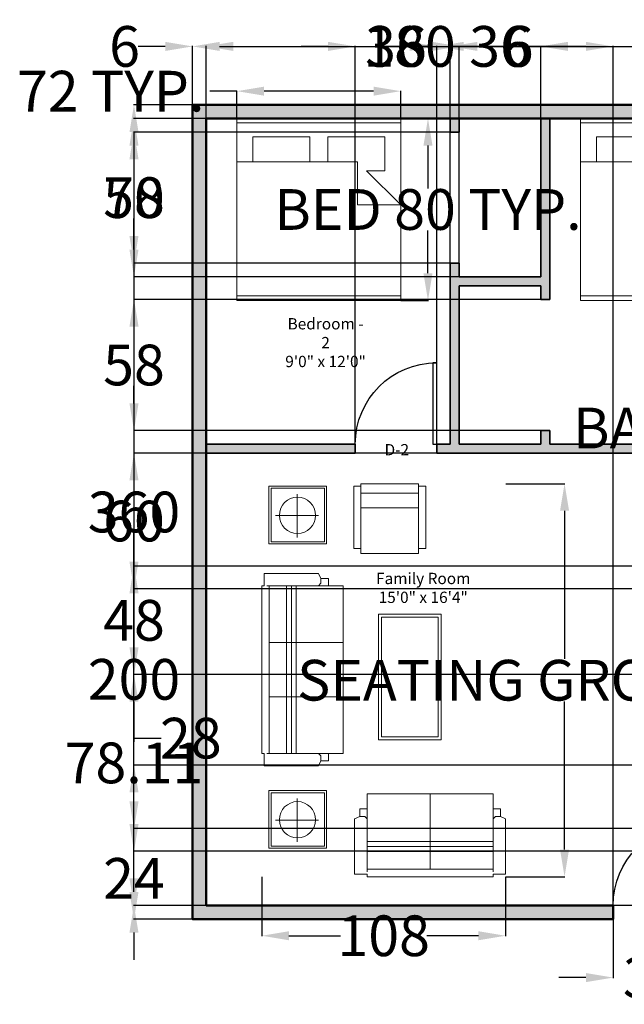
# Model space of a CAD drawing. Units: inches. Extents: x -478 to 256, y -93 to 343.
# Tile 1 of 5: x -478 to -211, y -93 to 343. Entities that reach past the tile are written whole.
import ezdxf

# ---------------------------------------------------------------- set-up
doc = ezdxf.new("R2010")
doc.units = ezdxf.units.IN
for name, color, linetype, lineweight in [('A-ANNO-DIMS', 2, 'Continuous', 18), ('A-ANNO-TEXT', 7, 'Continuous', 18), ('A-AREA-IDEN', 7, 'Continuous', 18), ('A-DOOR', 3, 'Continuous', 25), ('A-WALL-PATT', 8, 'Continuous', 13), ('Furniture', 2, 'Continuous', 18), ('Inner Wall', 5, 'Continuous', 35), ('Outer Wall', 1, 'Continuous', 50)]:
    doc.layers.add(name, color=color, linetype=linetype, lineweight=lineweight)
doc.styles.get("Standard").update_dxf_attribs({"font": 'arial.ttf'})
doc.dimstyles.get("Standard").update_dxf_attribs({"dimtxt": 18, "dimasz": 12, "dimexe": 0.18, "dimexo": 0.0625, "dimgap": 0.09, "dimtad": 0, "dimtih": 1, "dimtoh": 1, "dimdec": 0, "dimzin": 0, "dimdsep": 46, "dimlunit": 3, "dimtxsty": 'Standard', "dimcen": 0.09, "dimadec": 0, "dimazin": 0, "dimtfac": 1, "dimtdec": 0, "dimtofl": 0, "dimtmove": 0, "dimatfit": 3, "dimfxl": 1, "dimtolj": 1, "dimtzin": 0, "dimarcsym": 0})

# ---------------------------------------------------------------- blocks, each defined once
blk = doc.blocks.new('*U2')
for p, q in [((0, 0), (0, -4)), ((36, 0), (36, -4))]:
    blk.add_line(p, q)
blk.add_lwpolyline([(0, 0), (0, 36), (1.75, 36), (1.75, 0)], close=True)
blk.add_arc((0, 0), 36, 0, 90)
blk = doc.blocks.new('KING-00')
for p, q in [((-0.897, -0.947), (-0.897, 0.882)), ((0.602, 0.882), (0.602, -0.464)), ((1.034, -0.947), (1.034, 0.882)), ((0.602, 0.704), (0.881, 0.704)), ((0.881, 0.069), (0.881, 0.704)), ((0.602, 0.069), (0.881, 0.069)), ((0.881, -0.134), (0.602, -0.134)), ((0.881, -0.769), (0.881, -0.134)), ((0.119, -0.464), (0.119, -0.947)), ((0.602, -0.464), (0.119, -0.464)), ((0.119, -0.947), (0.5, -0.566)), ((0.5, -0.769), (0.5, -0.566)), ((0.5, -0.769), (0.881, -0.769))]:
    blk.add_line(p, q)
blk.add_lwpolyline([(-0.948, -0.947), (-0.948, 0.882), (1.084, 0.882), (1.084, -0.947)], close=True)
blk = doc.blocks.new('A$C518662A7')
for p, q in [((24.2, 2257.5), (574.2, 2257.5)), ((24.2, 1707.5), (24.2, 2257.5)), ((574.2, 2257.5), (574.2, 1707.5)), ((2927.5, 2257.5), (3477.5, 2257.5)), ((2927.5, 1707.5), (2927.5, 2257.5)), ((3477.5, 2257.5), (3477.5, 1707.5)), ((44.2, 2237.5), (554.2, 2237.5)), ((44.2, 1727.5), (44.2, 2237.5)), ((304.4, 2193.4), (304.4, 1783.3)), ((554.2, 2237.5), (554.2, 1727.5)), ((2947.5, 2237.5), (3457.5, 2237.5)), ((2947.5, 1727.5), (2947.5, 2237.5)), ((3207.6, 2193.4), (3207.6, 1783.3)), ((3457.5, 2237.5), (3457.5, 1727.5)), ((100.6, 1987.3), (512.6, 1987.3)), ((3003.8, 1987.3), (3415.8, 1987.3)), ((574.2, 1707.5), (24.2, 1707.5)), ((554.2, 1727.5), (44.2, 1727.5)), ((3477.5, 1707.5), (2927.5, 1707.5)), ((3457.5, 1727.5), (2947.5, 1727.5)), ((1243.6, 1213.6), (2443.6, 1213.6)), ((1243.6, 613.6), (1243.6, 1213.6)), ((1273.6, 1183.6), (2413.6, 1183.6)), ((1273.6, 643.6), (1273.6, 1183.6)), ((2413.6, 1183.6), (2413.6, 643.6)), ((2443.6, 1213.6), (2443.6, 613.6)), ((2443.6, 613.6), (1243.6, 613.6)), ((2413.6, 643.6), (1273.6, 643.6))]:
    blk.add_line(p, q)
at = {"linetype": 'ByBlock'}
for p, q in [((855.8, 2302.4), (973.4, 2302.4)), ((855.8, 1784.8), (855.8, 2302.4)), ((973.4, 2326), (2573.4, 2326)), ((973.4, 2302.4), (973.4, 2326)), ((973.4, 1784.8), (973.4, 2278.9)), ((973.4, 2255.4), (2573.4, 2255.4)), ((1514.6, 1549.5), (1514.6, 2255.4)), ((2032.3, 1549.5), (2032.3, 2255.4)), ((2573.4, 2326), (2573.4, 2302.4)), ((2573.4, 2302.4), (2691.1, 2302.4)), ((2573.4, 1784.8), (2573.4, 2278.9)), ((2691.1, 2302.4), (2691.1, 1784.8)), ((2573.4, 2090.7), (973.4, 2090.7)), ((2573.4, 2043.6), (973.4, 2043.6)), ((2573.4, 1996.5), (973.4, 1996.5)), ((902.9, 1761.3), (855.8, 1784.8)), ((949.9, 1761.3), (973.4, 1784.8)), ((973.4, 1690.7), (973.4, 1784.8)), ((2573.4, 1690.7), (2573.4, 1784.8)), ((2597, 1761.3), (2573.4, 1784.8)), ((2691.1, 1784.8), (2644, 1761.3)), ((902.9, 1761.3), (949.9, 1761.3)), ((902.9, 1690.7), (902.9, 1761.3)), ((973.4, 1690.7), (902.9, 1690.7)), ((973.4, 1549.5), (973.4, 1690.7)), ((2644, 1690.7), (2573.4, 1690.7)), ((2573.4, 1690.7), (2573.4, 1549.5)), ((2644, 1761.3), (2597, 1761.3)), ((2644, 1761.3), (2644, 1690.7)), ((2573.4, 1549.5), (973.4, 1549.5)), ((22.9, 1448.9), (22.9, 1380.2)), ((618.7, 1448.9), (22.9, 1448.9)), ((618.7, 1380.2), (618.7, 1448.9)), ((3173, 1392), (3197, 1440)), ((3197, 1440), (3725, 1440)), ((3725, 1440), (3725, 1320)), ((0, 1380.2), (0, 830.2)), ((664.6, 1380.2), (0, 1380.2)), ((91.7, 1380.2), (91.7, 830.2)), ((229.2, 830.2), (229.2, 1380.2)), ((664.6, 830.2), (664.6, 1380.2)), ((2957, 1320), (3101, 1320)), ((2957, 120), (2957, 1320)), ((3101, 1320), (3101, 1392)), ((3101, 1392), (3173, 1392)), ((3101, 1320), (3197, 1320)), ((3173, 1392), (3173, 1344)), ((3173, 1344), (3197, 1320)), ((3197, 1320), (3701, 1320)), ((3413, 120), (3413, 1320)), ((3461, 120), (3461, 1320)), ((3509, 120), (3509, 1320)), ((3677, 1320), (3677, 120)), ((3725, 1320), (3749, 1320)), ((3749, 1320), (3749, 120)), ((0, 830.2), (664.6, 830.2)), ((22.9, 830.2), (22.9, 761.4)), ((22.9, 761.4), (618.7, 761.4)), ((618.7, 761.4), (618.7, 830.2)), ((2957, 720), (3677, 720)), ((3101, 120), (2957, 120)), ((3101, 120), (3197, 120)), ((3101, 48), (3101, 120)), ((3173, 96), (3197, 120)), ((3173, 48), (3173, 96)), ((3197, 120), (3701, 120)), ((3749, 120), (3725, 120)), ((3725, 120), (3725, 0)), ((3173, 48), (3101, 48)), ((3197, 0), (3173, 48)), ((3725, 0), (3197, 0))]:
    blk.add_line(p, q, dxfattribs=at)
for centre in [(302.2, 1985.1), (3205.4, 1985.1)]:
    blk.add_circle(centre, 173.1)
blk = doc.blocks.new('*U14')
for p, q in [((0, 0), (0, -6)), ((36, 0), (36, -6))]:
    blk.add_line(p, q)
blk.add_lwpolyline([(0, 0), (0, 36), (1.75, 36), (1.75, 0)], close=True)
blk.add_arc((0, 0), 36, 0, 90)
blk = doc.blocks.new('*D15')
at = {"layer": 'A-ANNO-DIMS', "color": 0, "lineweight": -2, "transparency": 16777216}
for p, q in [((-309.72, 298.84), (-297.53, 298.84)), ((-297.71, 286.84), (-297.71, 267.89)), ((-297.71, 230.37), (-297.71, 249.32)), ((-309.72, 218.37), (-297.53, 218.37))]:
    blk.add_line(p, q, dxfattribs=at)
at = {"layer": 'A-ANNO-DIMS', "color": 0, "transparency": 16777216}
for points in [[(-299.71, 286.84), (-295.71, 286.84), (-297.71, 298.84)], [(-299.71, 230.37), (-295.71, 230.37), (-297.71, 218.37)]]:
    blk.add_solid(points, dxfattribs=at)
at = {"layer": 'Defpoints', "color": 0, "transparency": 16777216}
for p in [(-309.78, 298.84), (-297.71, 298.84), (-309.78, 218.37)]:
    blk.add_point(p, dxfattribs=at)
at = {"layer": 'A-ANNO-DIMS', "color": 0, "transparency": 16777216, "insert": (-297.71, 258.6), "char_height": 18, "attachment_point": 5}
blk.add_mtext('\\A1;BED 80 TYP.', dxfattribs=at)
blk = doc.blocks.new('*D16')
at = {"layer": 'A-ANNO-DIMS', "color": 0, "lineweight": -2, "transparency": 16777216}
for p, q in [((-382.2, 310.91), (-394.2, 310.91)), ((-382.2, 298.9), (-382.2, 311.09)), ((-321.78, 310.91), (-370.2, 310.91)), ((-309.78, 298.9), (-309.78, 311.09))]:
    blk.add_line(p, q, dxfattribs=at)
at = {"layer": 'A-ANNO-DIMS', "color": 0, "transparency": 16777216}
for points in [[(-370.2, 312.91), (-370.2, 308.91), (-382.2, 310.91)], [(-321.78, 312.91), (-321.78, 308.91), (-309.78, 310.91)]]:
    blk.add_solid(points, dxfattribs=at)
at = {"layer": 'Defpoints', "color": 0, "transparency": 16777216}
for p in [(-382.2, 310.91), (-382.2, 298.84), (-309.78, 298.84)]:
    blk.add_point(p, dxfattribs=at)
at = {"layer": 'A-ANNO-DIMS', "color": 0, "transparency": 16777216, "insert": (-438.03, 310.91), "char_height": 18, "attachment_point": 5}
blk.add_mtext('\\A1;72 TYP.', dxfattribs=at)
blk = doc.blocks.new('*D25')
at = {"layer": 'A-ANNO-DIMS', "color": 0, "lineweight": -2, "transparency": 16777216}
for p, q in [((-116.04, 214.73), (-116.04, 226.73)), ((-118.49, 202.73), (-115.86, 202.73)), ((-118.49, 185.95), (-115.86, 185.95)), ((-116.04, 173.95), (-116.04, 161.95)), ((-116.04, 161.95), (-128.04, 161.95))]:
    blk.add_line(p, q, dxfattribs=at)
at = {"layer": 'A-ANNO-DIMS', "color": 0, "transparency": 16777216}
for points in [[(-118.04, 214.73), (-114.04, 214.73), (-116.04, 202.73)], [(-118.04, 173.95), (-114.04, 173.95), (-116.04, 185.95)]]:
    blk.add_solid(points, dxfattribs=at)
at = {"layer": 'Defpoints', "color": 0, "transparency": 16777216}
for p in [(-118.56, 202.73), (-118.56, 185.95), (-116.04, 185.95)]:
    blk.add_point(p, dxfattribs=at)
at = {"layer": 'A-ANNO-DIMS', "color": 0, "transparency": 16777216, "insert": (-181.85, 161.95), "char_height": 18, "attachment_point": 5}
blk.add_mtext('\\A1;BASIN 17', dxfattribs=at)
blk = doc.blocks.new('*D29')
at = {"layer": 'A-ANNO-DIMS', "color": 0, "lineweight": -2, "transparency": 16777216}
for p, q in [((-263.32, 137.36), (-237.13, 137.36)), ((-237.31, 125.36), (-237.31, 59.86)), ((-237.31, -24.45), (-237.31, 41.05)), ((-263.32, -36.45), (-237.13, -36.45))]:
    blk.add_line(p, q, dxfattribs=at)
at = {"layer": 'A-ANNO-DIMS', "color": 0, "transparency": 16777216}
for points in [[(-239.31, 125.36), (-235.31, 125.36), (-237.31, 137.36)], [(-239.31, -24.45), (-235.31, -24.45), (-237.31, -36.45)]]:
    blk.add_solid(points, dxfattribs=at)
at = {"layer": 'Defpoints', "color": 0, "transparency": 16777216}
for p in [(-263.38, 137.36), (-263.38, -36.45), (-237.31, -36.45)]:
    blk.add_point(p, dxfattribs=at)
at = {"layer": 'A-ANNO-DIMS', "color": 0, "transparency": 16777216, "insert": (-237.31, 50.46), "char_height": 18, "attachment_point": 5}
blk.add_mtext('\\A1;SEATING GROUP 174', dxfattribs=at)
blk = doc.blocks.new('*D30')
at = {"layer": 'A-ANNO-DIMS', "color": 0, "lineweight": -2, "transparency": 16777216}
for p, q in [((-371.22, -36.51), (-371.22, -62.7)), ((-263.38, -36.51), (-263.38, -62.7)), ((-359.22, -62.52), (-336.45, -62.52)), ((-275.38, -62.52), (-298.15, -62.52))]:
    blk.add_line(p, q, dxfattribs=at)
at = {"layer": 'A-ANNO-DIMS', "color": 0, "transparency": 16777216}
for points in [[(-359.22, -60.52), (-359.22, -64.52), (-371.22, -62.52)], [(-275.38, -60.52), (-275.38, -64.52), (-263.38, -62.52)]]:
    blk.add_solid(points, dxfattribs=at)
at = {"layer": 'Defpoints', "color": 0, "transparency": 16777216}
for p in [(-371.22, -36.45), (-263.38, -36.45), (-371.22, -62.52)]:
    blk.add_point(p, dxfattribs=at)
at = {"layer": 'A-ANNO-DIMS', "color": 0, "transparency": 16777216, "insert": (-317.3, -62.52), "char_height": 18, "attachment_point": 5}
blk.add_mtext('\\A1;108', dxfattribs=at)
blk = doc.blocks.new('*D31')
at = {"layer": 'A-ANNO-DIMS', "color": 0, "lineweight": -2, "transparency": 16777216}
for p, q in [((-401.86, 304.9), (-401.86, 330.89)), ((78.14, 304.9), (78.14, 330.89)), ((-389.86, 330.71), (-182.16, 330.71)), ((66.14, 330.71), (-141.55, 330.71))]:
    blk.add_line(p, q, dxfattribs=at)
at = {"layer": 'A-ANNO-DIMS', "color": 0, "transparency": 16777216}
for points in [[(-389.86, 332.71), (-389.86, 328.71), (-401.86, 330.71)], [(66.14, 332.71), (66.14, 328.71), (78.14, 330.71)]]:
    blk.add_solid(points, dxfattribs=at)
at = {"layer": 'Defpoints', "color": 0, "transparency": 16777216}
for p in [(78.14, 330.71), (-401.86, 304.84), (78.14, 304.84)]:
    blk.add_point(p, dxfattribs=at)
at = {"layer": 'A-ANNO-DIMS', "color": 0, "transparency": 16777216, "insert": (-161.86, 330.71), "char_height": 18, "attachment_point": 5}
blk.add_mtext('\\A1;480', dxfattribs=at)
blk = doc.blocks.new('*D32')
at = {"layer": 'A-ANNO-DIMS', "color": 0, "lineweight": -2, "transparency": 16777216}
for p, q in [((-401.92, 304.84), (-427.9, 304.84)), ((-427.72, 292.84), (-427.72, 134.13)), ((-427.72, -43.16), (-427.72, 115.55)), ((-401.92, -55.16), (-427.9, -55.16))]:
    blk.add_line(p, q, dxfattribs=at)
at = {"layer": 'A-ANNO-DIMS', "color": 0, "transparency": 16777216}
for points in [[(-429.72, 292.84), (-425.72, 292.84), (-427.72, 304.84)], [(-429.72, -43.16), (-425.72, -43.16), (-427.72, -55.16)]]:
    blk.add_solid(points, dxfattribs=at)
at = {"layer": 'Defpoints', "color": 0, "transparency": 16777216}
for p in [(-427.72, 304.84), (-401.86, 304.84), (-401.86, -55.16)]:
    blk.add_point(p, dxfattribs=at)
at = {"layer": 'A-ANNO-DIMS', "color": 0, "transparency": 16777216, "insert": (-427.72, 124.84), "char_height": 18, "attachment_point": 5}
blk.add_mtext('\\A1;360', dxfattribs=at)
blk = doc.blocks.new('*D33')
at = {"layer": 'A-ANNO-DIMS', "color": 0, "lineweight": -2, "transparency": 16777216}
for p, q in [((-395.86, -49.1), (-395.86, 330.89)), ((-215.86, -49.1), (-215.86, 330.89)), ((-383.86, 330.71), (-324.95, 330.71)), ((-227.86, 330.71), (-286.76, 330.71))]:
    blk.add_line(p, q, dxfattribs=at)
at = {"layer": 'A-ANNO-DIMS', "color": 0, "transparency": 16777216}
for points in [[(-383.86, 332.71), (-383.86, 328.71), (-395.86, 330.71)], [(-227.86, 332.71), (-227.86, 328.71), (-215.86, 330.71)]]:
    blk.add_solid(points, dxfattribs=at)
at = {"layer": 'Defpoints', "color": 0, "transparency": 16777216}
for p in [(-215.86, 330.71), (-395.86, -49.16), (-215.86, -49.16)]:
    blk.add_point(p, dxfattribs=at)
at = {"layer": 'A-ANNO-DIMS', "color": 0, "transparency": 16777216, "insert": (-305.86, 330.71), "char_height": 18, "attachment_point": 5}
blk.add_mtext('\\A1;180', dxfattribs=at)
blk = doc.blocks.new('*D34')
at = {"layer": 'A-ANNO-DIMS', "color": 0, "lineweight": -2, "transparency": 16777216}
for p, q in [((-215.855811, -55.221403), (-215.855811, -81.203903)), ((-179.855811, -55.221403), (-179.855811, -81.203903)), ((-227.855811, -81.023903), (-239.855811, -81.023903)), ((-167.855811, -81.023903), (-155.855811, -81.023903))]:
    blk.add_line(p, q, dxfattribs=at)
at = {"layer": 'A-ANNO-DIMS', "color": 0, "transparency": 16777216}
for points in [[(-227.855811, -79.023903), (-227.855811, -83.023903), (-215.855811, -81.023903)], [(-167.855811, -79.023903), (-167.855811, -83.023903), (-179.855811, -81.023903)]]:
    blk.add_solid(points, dxfattribs=at)
at = {"layer": 'Defpoints', "color": 0, "transparency": 16777216}
for p in [(-215.855811, -55.158903), (-179.855811, -55.158903), (-179.855811, -81.023903)]:
    blk.add_point(p, dxfattribs=at)
at = {"layer": 'A-ANNO-DIMS', "color": 0, "transparency": 16777216, "insert": (-197.855811, -81.023903), "char_height": 18, "attachment_point": 5}
blk.add_mtext('\\A1;36', dxfattribs=at)
blk = doc.blocks.new('*D36')
at = {"layer": 'A-ANNO-DIMS', "color": 0, "lineweight": -2, "transparency": 16777216}
for p, q in [((-395.92, 150.84), (-427.9, 150.84)), ((-427.72, 138.84), (-427.72, 60.12)), ((-427.72, -37.16), (-427.72, 41.56)), ((-395.92, -49.16), (-427.9, -49.16))]:
    blk.add_line(p, q, dxfattribs=at)
at = {"layer": 'A-ANNO-DIMS', "color": 0, "transparency": 16777216}
for points in [[(-429.72, 138.84), (-425.72, 138.84), (-427.72, 150.84)], [(-429.72, -37.16), (-425.72, -37.16), (-427.72, -49.16)]]:
    blk.add_solid(points, dxfattribs=at)
at = {"layer": 'Defpoints', "color": 0, "transparency": 16777216}
for p in [(-427.72, 150.84), (-395.86, 150.84), (-395.86, -49.16)]:
    blk.add_point(p, dxfattribs=at)
at = {"layer": 'A-ANNO-DIMS', "color": 0, "transparency": 16777216, "insert": (-427.72, 50.84), "char_height": 18, "attachment_point": 5}
blk.add_mtext('\\A1;200', dxfattribs=at)
blk = doc.blocks.new('*D37')
at = {"layer": 'A-ANNO-DIMS', "color": 0, "lineweight": -2, "transparency": 16777216}
for p, q in [((-283.855811, 228.903597), (-283.855811, 330.886097)), ((-247.855811, 228.903597), (-247.855811, 330.886097)), ((-295.855811, 330.706097), (-307.855811, 330.706097)), ((-235.855811, 330.706097), (-223.855811, 330.706097))]:
    blk.add_line(p, q, dxfattribs=at)
at = {"layer": 'A-ANNO-DIMS', "color": 0, "transparency": 16777216}
for points in [[(-295.855811, 332.706097), (-295.855811, 328.706097), (-283.855811, 330.706097)], [(-235.855811, 332.706097), (-235.855811, 328.706097), (-247.855811, 330.706097)]]:
    blk.add_solid(points, dxfattribs=at)
at = {"layer": 'Defpoints', "color": 0, "transparency": 16777216}
for p in [(-247.855811, 330.706097), (-283.855811, 228.841097), (-247.855811, 228.841097)]:
    blk.add_point(p, dxfattribs=at)
at = {"layer": 'A-ANNO-DIMS', "color": 0, "transparency": 16777216, "insert": (-265.855811, 330.706097), "char_height": 18, "attachment_point": 5}
blk.add_mtext('\\A1;36', dxfattribs=at)
blk = doc.blocks.new('*D38')
at = {"layer": 'A-ANNO-DIMS', "color": 0, "lineweight": -2, "transparency": 16777216}
for p, q in [((-247.92, 298.84), (-427.9, 298.84)), ((-427.72, 286.84), (-427.72, 273.12)), ((-427.72, 240.84), (-427.72, 254.56)), ((-247.92, 228.84), (-427.9, 228.84))]:
    blk.add_line(p, q, dxfattribs=at)
at = {"layer": 'A-ANNO-DIMS', "color": 0, "transparency": 16777216}
for points in [[(-429.72, 286.84), (-425.72, 286.84), (-427.72, 298.84)], [(-429.72, 240.84), (-425.72, 240.84), (-427.72, 228.84)]]:
    blk.add_solid(points, dxfattribs=at)
at = {"layer": 'Defpoints', "color": 0, "transparency": 16777216}
for p in [(-427.72, 298.84), (-247.86, 298.84), (-247.86, 228.84)]:
    blk.add_point(p, dxfattribs=at)
at = {"layer": 'A-ANNO-DIMS', "color": 0, "transparency": 16777216, "insert": (-427.72, 263.84), "char_height": 18, "attachment_point": 5}
blk.add_mtext('\\A1;70', dxfattribs=at)
blk = doc.blocks.new('*D42')
at = {"layer": 'A-ANNO-DIMS', "color": 0, "lineweight": -2, "transparency": 16777216}
for p, q in [((-329.855811, 154.903597), (-329.855811, 330.886097)), ((-293.855811, 154.903597), (-293.855811, 330.886097)), ((-341.855811, 330.706097), (-353.855811, 330.706097)), ((-281.855811, 330.706097), (-269.855811, 330.706097))]:
    blk.add_line(p, q, dxfattribs=at)
at = {"layer": 'A-ANNO-DIMS', "color": 0, "transparency": 16777216}
for points in [[(-341.855811, 332.706097), (-341.855811, 328.706097), (-329.855811, 330.706097)], [(-281.855811, 332.706097), (-281.855811, 328.706097), (-293.855811, 330.706097)]]:
    blk.add_solid(points, dxfattribs=at)
at = {"layer": 'Defpoints', "color": 0, "transparency": 16777216}
for p in [(-293.855811, 330.706097), (-329.855811, 154.841097), (-293.855811, 154.841097)]:
    blk.add_point(p, dxfattribs=at)
at = {"layer": 'A-ANNO-DIMS', "color": 0, "transparency": 16777216, "insert": (-311.855811, 330.706097), "char_height": 18, "attachment_point": 5}
blk.add_mtext('\\A1;36', dxfattribs=at)
blk = doc.blocks.new('*D43')
at = {"layer": 'A-ANNO-DIMS', "color": 0, "lineweight": -2, "transparency": 16777216}
for p, q in [((-293.86, 154.9), (-293.86, 330.89)), ((-287.86, 154.9), (-287.86, 330.89)), ((-305.86, 330.71), (-317.86, 330.71)), ((-275.86, 330.71), (-263.86, 330.71))]:
    blk.add_line(p, q, dxfattribs=at)
at = {"layer": 'A-ANNO-DIMS', "color": 0, "transparency": 16777216}
for points in [[(-305.86, 332.71), (-305.86, 328.71), (-293.86, 330.71)], [(-275.86, 332.71), (-275.86, 328.71), (-287.86, 330.71)]]:
    blk.add_solid(points, dxfattribs=at)
at = {"layer": 'Defpoints', "color": 0, "transparency": 16777216}
for p in [(-287.86, 330.71), (-293.86, 154.84), (-287.86, 154.84)]:
    blk.add_point(p, dxfattribs=at)
at = {"layer": 'A-ANNO-DIMS', "color": 0, "transparency": 16777216, "insert": (-257.82, 330.71), "char_height": 18, "attachment_point": 5}
blk.add_mtext('\\A1;6', dxfattribs=at)
blk = doc.blocks.new('*D52')
at = {"layer": 'A-ANNO-DIMS', "color": 0, "lineweight": -2, "transparency": 16777216}
for p, q in [((-427.72, 12.84), (-427.72, 24.84)), ((-427.72, 24.84), (-415.72, 24.84)), ((0.08, 12.84), (-427.9, 12.84)), ((-427.72, -3.16), (-427.72, 0.84)), ((0.08, -15.16), (-427.9, -15.16))]:
    blk.add_line(p, q, dxfattribs=at)
at = {"layer": 'A-ANNO-DIMS', "color": 0, "transparency": 16777216}
for points in [[(-429.72, 0.84), (-425.72, 0.84), (-427.72, 12.84)], [(-429.72, -3.16), (-425.72, -3.16), (-427.72, -15.16)]]:
    blk.add_solid(points, dxfattribs=at)
at = {"layer": 'Defpoints', "color": 0, "transparency": 16777216}
for p in [(-427.72, 12.84), (0.14, 12.84), (0.14, -15.16)]:
    blk.add_point(p, dxfattribs=at)
at = {"layer": 'A-ANNO-DIMS', "color": 0, "transparency": 16777216, "insert": (-402.57, 24.84), "char_height": 18, "attachment_point": 5}
blk.add_mtext('\\A1;28', dxfattribs=at)
blk = doc.blocks.new('*D54')
at = {"layer": 'A-ANNO-DIMS', "color": 0, "lineweight": -2, "transparency": 16777216}
for p, q in [((-106.35, 100.95), (-427.9, 100.95)), ((-427.72, 88.95), (-427.72, 86.23)), ((-427.72, 64.95), (-427.72, 67.67)), ((-106.35, 52.95), (-427.9, 52.95))]:
    blk.add_line(p, q, dxfattribs=at)
at = {"layer": 'A-ANNO-DIMS', "color": 0, "transparency": 16777216}
for points in [[(-429.72, 88.95), (-425.72, 88.95), (-427.72, 100.95)], [(-429.72, 64.95), (-425.72, 64.95), (-427.72, 52.95)]]:
    blk.add_solid(points, dxfattribs=at)
at = {"layer": 'Defpoints', "color": 0, "transparency": 16777216}
for p in [(-427.72, 100.95), (-106.28, 100.95), (-106.28, 52.95)]:
    blk.add_point(p, dxfattribs=at)
at = {"layer": 'A-ANNO-DIMS', "color": 0, "transparency": 16777216, "insert": (-427.72, 76.95), "char_height": 18, "attachment_point": 5}
blk.add_mtext('\\A1;48', dxfattribs=at)
blk = doc.blocks.new('*D55')
at = {"layer": 'A-ANNO-DIMS', "color": 0, "lineweight": -2, "transparency": 16777216}
for p, q in [((-401.86, 304.9), (-401.86, 330.89)), ((-395.86, 298.9), (-395.86, 330.89)), ((-413.86, 330.71), (-425.86, 330.71)), ((-383.86, 330.71), (-371.86, 330.71))]:
    blk.add_line(p, q, dxfattribs=at)
at = {"layer": 'A-ANNO-DIMS', "color": 0, "transparency": 16777216}
for points in [[(-413.86, 332.71), (-413.86, 328.71), (-401.86, 330.71)], [(-383.86, 332.71), (-383.86, 328.71), (-395.86, 330.71)]]:
    blk.add_solid(points, dxfattribs=at)
at = {"layer": 'Defpoints', "color": 0, "transparency": 16777216}
for p in [(-401.86, 330.71), (-401.86, 304.84), (-395.86, 298.84)]:
    blk.add_point(p, dxfattribs=at)
at = {"layer": 'A-ANNO-DIMS', "color": 0, "transparency": 16777216, "insert": (-431.89, 330.71), "char_height": 18, "attachment_point": 5}
blk.add_mtext('\\A1;6', dxfattribs=at)
blk = doc.blocks.new('*D58')
at = {"layer": 'A-ANNO-DIMS', "color": 0, "lineweight": -2, "transparency": 16777216}
for p, q in [((-427.720811, -13.158903), (-427.720811, -1.158903)), ((-99.918311, -25.158903), (-427.900811, -25.158903)), ((-99.918311, -49.158903), (-427.900811, -49.158903)), ((-427.720811, -61.158903), (-427.720811, -73.158903))]:
    blk.add_line(p, q, dxfattribs=at)
at = {"layer": 'A-ANNO-DIMS', "color": 0, "transparency": 16777216}
for points in [[(-429.720811, -13.158903), (-425.720811, -13.158903), (-427.720811, -25.158903)], [(-429.720811, -61.158903), (-425.720811, -61.158903), (-427.720811, -49.158903)]]:
    blk.add_solid(points, dxfattribs=at)
at = {"layer": 'Defpoints', "color": 0, "transparency": 16777216}
for p in [(-427.720811, -25.158903), (-99.855811, -25.158903), (-99.855811, -49.158903)]:
    blk.add_point(p, dxfattribs=at)
at = {"layer": 'A-ANNO-DIMS', "color": 0, "transparency": 16777216, "insert": (-427.720811, -37.158903), "char_height": 18, "attachment_point": 5}
blk.add_mtext('\\A1;24', dxfattribs=at)
blk = doc.blocks.new('*D61')
at = {"layer": 'A-ANNO-DIMS', "color": 0, "lineweight": -2, "transparency": 16777216}
for p, q in [((-106.35, 52.95), (-427.9, 52.95)), ((-427.72, 40.95), (-427.72, 23.18)), ((-427.72, -13.16), (-427.72, 4.61)), ((-99.92, -25.16), (-427.9, -25.16))]:
    blk.add_line(p, q, dxfattribs=at)
at = {"layer": 'A-ANNO-DIMS', "color": 0, "transparency": 16777216}
for points in [[(-429.72, 40.95), (-425.72, 40.95), (-427.72, 52.95)], [(-429.72, -13.16), (-425.72, -13.16), (-427.72, -25.16)]]:
    blk.add_solid(points, dxfattribs=at)
at = {"layer": 'Defpoints', "color": 0, "transparency": 16777216}
for p in [(-427.72, 52.95), (-106.28, 52.95), (-99.86, -25.16)]:
    blk.add_point(p, dxfattribs=at)
at = {"layer": 'A-ANNO-DIMS', "color": 0, "transparency": 16777216, "insert": (-427.72, 13.9), "char_height": 18, "attachment_point": 5}
blk.add_mtext('\\A1;78.11', dxfattribs=at)
blk = doc.blocks.new('*D63')
at = {"layer": 'A-ANNO-DIMS', "color": 0, "lineweight": -2, "transparency": 16777216}
for p, q in [((-287.92, 292.84), (-427.9, 292.84)), ((-427.72, 280.84), (-427.72, 273.12)), ((-427.72, 246.84), (-427.72, 254.56)), ((-287.92, 234.84), (-427.9, 234.84))]:
    blk.add_line(p, q, dxfattribs=at)
at = {"layer": 'A-ANNO-DIMS', "color": 0, "transparency": 16777216}
for points in [[(-429.72, 280.84), (-425.72, 280.84), (-427.72, 292.84)], [(-429.72, 246.84), (-425.72, 246.84), (-427.72, 234.84)]]:
    blk.add_solid(points, dxfattribs=at)
at = {"layer": 'Defpoints', "color": 0, "transparency": 16777216}
for p in [(-427.72, 292.84), (-287.86, 292.84), (-287.86, 234.84)]:
    blk.add_point(p, dxfattribs=at)
at = {"layer": 'A-ANNO-DIMS', "color": 0, "transparency": 16777216, "insert": (-427.72, 263.84), "char_height": 18, "attachment_point": 5}
blk.add_mtext('\\A1;58', dxfattribs=at)
blk = doc.blocks.new('*D64')
at = {"layer": 'A-ANNO-DIMS', "color": 0, "lineweight": -2, "transparency": 16777216}
for p, q in [((-247.92, 218.84), (-427.9, 218.84)), ((-427.72, 206.84), (-427.72, 199.12)), ((-427.72, 172.84), (-427.72, 180.56)), ((-247.92, 160.84), (-427.9, 160.84))]:
    blk.add_line(p, q, dxfattribs=at)
at = {"layer": 'A-ANNO-DIMS', "color": 0, "transparency": 16777216}
for points in [[(-429.72, 206.84), (-425.72, 206.84), (-427.72, 218.84)], [(-429.72, 172.84), (-425.72, 172.84), (-427.72, 160.84)]]:
    blk.add_solid(points, dxfattribs=at)
at = {"layer": 'Defpoints', "color": 0, "transparency": 16777216}
for p in [(-427.72, 218.84), (-247.86, 218.84), (-247.86, 160.84)]:
    blk.add_point(p, dxfattribs=at)
at = {"layer": 'A-ANNO-DIMS', "color": 0, "transparency": 16777216, "insert": (-427.72, 189.84), "char_height": 18, "attachment_point": 5}
blk.add_mtext('\\A1;58', dxfattribs=at)
blk = doc.blocks.new('*D66')
at = {"layer": 'A-ANNO-DIMS', "color": 0, "lineweight": -2, "transparency": 16777216}
for p, q in [((24.08, 150.84), (-427.9, 150.84)), ((-427.72, 138.84), (-427.72, 130.12)), ((-427.72, 102.84), (-427.72, 111.56)), ((24.08, 90.84), (-427.9, 90.84))]:
    blk.add_line(p, q, dxfattribs=at)
at = {"layer": 'A-ANNO-DIMS', "color": 0, "transparency": 16777216}
for points in [[(-429.72, 138.84), (-425.72, 138.84), (-427.72, 150.84)], [(-429.72, 102.84), (-425.72, 102.84), (-427.72, 90.84)]]:
    blk.add_solid(points, dxfattribs=at)
at = {"layer": 'Defpoints', "color": 0, "transparency": 16777216}
for p in [(-427.72, 150.84), (24.14, 150.84), (24.14, 90.84)]:
    blk.add_point(p, dxfattribs=at)
at = {"layer": 'A-ANNO-DIMS', "color": 0, "transparency": 16777216, "insert": (-427.72, 120.84), "char_height": 18, "attachment_point": 5}
blk.add_mtext('\\A1;60', dxfattribs=at)
blk = doc.blocks.new('*D68')
at = {"layer": 'A-ANNO-DIMS', "color": 0, "lineweight": -2, "transparency": 16777216}
for p, q in [((-427.720811, -13.158903), (-427.720811, -1.158903)), ((72.081689, -25.158903), (-427.900811, -25.158903)), ((72.081689, -49.158903), (-427.900811, -49.158903)), ((-427.720811, -61.158903), (-427.720811, -73.158903))]:
    blk.add_line(p, q, dxfattribs=at)
at = {"layer": 'A-ANNO-DIMS', "color": 0, "transparency": 16777216}
for points in [[(-429.720811, -13.158903), (-425.720811, -13.158903), (-427.720811, -25.158903)], [(-429.720811, -61.158903), (-425.720811, -61.158903), (-427.720811, -49.158903)]]:
    blk.add_solid(points, dxfattribs=at)
at = {"layer": 'Defpoints', "color": 0, "transparency": 16777216}
for p in [(-427.720811, -25.158903), (72.144189, -25.158903), (72.144189, -49.158903)]:
    blk.add_point(p, dxfattribs=at)
at = {"layer": 'A-ANNO-DIMS', "color": 0, "transparency": 16777216, "insert": (-427.720811, -37.158903), "char_height": 18, "attachment_point": 5}
blk.add_mtext('\\A1;24', dxfattribs=at)

msp = doc.modelspace()

# ---------------------------------------------------------------- hatches: boundary and pattern name
at = {"layer": 'A-WALL-PATT'}
h = msp.add_hatch(color=256, dxfattribs=at)
h.dxf.hatch_style = 1
h.paths.add_polyline_path([(-395.856, 298.841), (72.144, 298.841), (72.144, 20.841), (78.144, 20.841), (78.144, 304.841), (-401.856, 304.841), (-401.856, -55.159), (-215.856, -55.159), (-215.856, -49.159), (-395.856, -49.159)])
h.paths.add_polyline_path([(78.144, -15.159), (72.144, -15.159), (72.144, -49.159), (-179.856, -49.159), (-179.856, -55.159), (78.144, -55.159)], flags=17)
h = msp.add_hatch(color=256, dxfattribs=at)
h.dxf.hatch_style = 1
h.paths.add_polyline_path([(-329.856, 154.841), (-395.856, 154.841), (-395.856, 150.841), (-329.856, 150.841)])
h.paths.add_polyline_path([(-177.856, 154.841), (-243.856, 154.841), (-243.856, 160.841), (-247.856, 160.841), (-247.856, 154.841), (-283.856, 154.841), (-283.856, 224.841), (-247.856, 224.841), (-247.856, 218.841), (-243.856, 218.841), (-243.856, 298.841), (-247.856, 298.841), (-247.856, 228.841), (-283.856, 228.841), (-283.856, 234.841), (-287.856, 234.841), (-287.856, 154.841), (-293.856, 154.841), (-293.856, 150.841), (-177.856, 150.841)])
h.paths.add_polyline_path([(-283.856, 298.841), (-287.856, 298.841), (-287.856, 292.841), (-283.856, 292.841)], flags=17)
h.paths.add_polyline_path([(-131.856, 298.841), (-135.856, 298.841), (-135.856, 154.841), (-141.856, 154.841), (-141.856, 150.841), (-117.856, 150.841), (-117.856, 154.841), (-131.856, 154.841)])
h.paths.add_polyline_path([(-79.856, 298.841), (-83.856, 298.841), (-83.856, 154.841), (-89.856, 154.841), (-89.856, 150.841), (-73.856, 150.841), (-73.856, 154.841), (-79.856, 154.841)])
h.paths.add_polyline_path([(32.144, 154.841), (-33.856, 154.841), (-33.856, 150.841), (-3.856, 150.841), (-3.856, 12.841), (0.144, 12.841), (0.144, 62.841), (72.144, 62.841), (72.144, 66.841), (0.144, 66.841), (0.144, 150.841), (32.144, 150.841)])
h.paths.add_polyline_path([(72.144, 154.841), (60.144, 154.841), (60.144, 150.841), (72.144, 150.841)], flags=17)
h.paths.add_polyline_path([(6.144, -21.159), (0.144, -21.159), (0.144, -15.159), (-3.856, -15.159), (-3.856, -49.159), (0.144, -49.159), (0.144, -25.159), (6.144, -25.159)])
h.paths.add_polyline_path([(72.144, -21.159), (66.144, -21.159), (66.144, -25.159), (72.144, -25.159)])

# ---------------------------------------------------------------- linework, layer by layer
at = {"layer": 'Inner Wall'}
for p, q in [((-287.856, 292.841), (-287.856, 298.841)), ((-283.856, 292.841), (-283.856, 298.841)), ((-247.856, 298.841), (-247.856, 228.841)), ((-243.856, 298.841), (-243.856, 218.841)), ((-287.856, 292.841), (-283.856, 292.841)), ((-287.856, 154.841), (-287.856, 234.841)), ((-287.856, 234.841), (-283.856, 234.841)), ((-283.856, 228.841), (-283.856, 234.841)), ((-283.856, 228.841), (-247.856, 228.841)), ((-283.856, 154.841), (-283.856, 224.841)), ((-283.856, 224.841), (-247.856, 224.841)), ((-247.856, 224.841), (-247.856, 218.841)), ((-247.856, 218.841), (-243.856, 218.841)), ((-247.856, 160.841), (-243.856, 160.841)), ((-247.856, 160.841), (-247.856, 154.841)), ((-243.856, 160.841), (-243.856, 154.841)), ((-395.856, 154.841), (-329.856, 154.841)), ((-329.856, 150.841), (-329.856, 154.841)), ((-293.856, 150.841), (-293.856, 154.841)), ((-293.856, 154.841), (-287.856, 154.841)), ((-283.856, 154.841), (-247.856, 154.841)), ((-243.856, 154.841), (-177.856, 154.841)), ((-395.856, 150.841), (-329.856, 150.841)), ((-293.856, 150.841), (-177.856, 150.841))]:
    msp.add_line(p, q, dxfattribs=at)
at = {"layer": 'Outer Wall'}
for p, q in [((-395.856, 298.841), (72.144, 298.841)), ((-395.856, -49.159), (-395.856, 298.841)), ((-215.856, -49.159), (-395.856, -49.159)), ((-215.856, -55.159), (-215.856, -49.159))]:
    msp.add_line(p, q, dxfattribs=at)
msp.add_lwpolyline([(-215.856, -55.159), (-401.856, -55.159), (-401.856, 304.841), (78.144, 304.841), (78.144, 20.841)], dxfattribs=at)

# ---------------------------------------------------------------- block references
at = {"layer": 'A-DOOR', "xscale": -1}
for name, p in [('*U2', (-293.856, 154.841)), ('*U14', (-179.856, -49.159))]:
    msp.add_blockref(name, p, dxfattribs=at)
at = {"layer": 'Furniture'}
for name, p, xscale, yscale, zscale, rotation in [('KING-00', (-347.282, 255.892), 39.60249106241186, 39.60249106241186, 39.60249106241186, 89.99999999999999), ('KING-00', (-195.282, 255.892), 39.60249106241186, 39.60249106241186, 39.60249106241186, 89.99999999999999), ('A$C518662A7', (-263.384, 137.358), -0.0463602785226084, 0.0463602785226084, 0.0463602785226084, 90)]:
    msp.add_blockref(name, p, dxfattribs=dict(at, xscale=xscale, yscale=yscale, zscale=zscale, rotation=rotation))

# ---------------------------------------------------------------- texts
at = {"layer": 'A-ANNO-TEXT', "insert": (-301.989, 154.888), "char_height": 5, "attachment_point": 3}
msp.add_mtext_dynamic_manual_height_columns('\\pxqc;{\\fTimes New Roman|b0|i0|c0|p18;D-2}', width=19.01487, gutter_width=12.5, heights=[0], dxfattribs=at)
at = {"layer": 'A-AREA-IDEN', "char_height": 5, "attachment_point": 3}
for s, width, insert in [('\\pxqc;{\\fTimes New Roman|b0|i0|c0|p18;Bedroom - 2\\P9\'0" x 12\'0"}', 37.20338, (-324.393, 210.568)), ('\\pxqc;{\\fTimes New Roman|b0|i0|c0|p18;Family Room\\P15\'0" x 16\'4"}', 53.31763, (-273.149, 97.954))]:
    msp.add_mtext_dynamic_manual_height_columns(s, width=width, gutter_width=12.5, heights=[0], dxfattribs=dict(at, insert=insert))

# ---------------------------------------------------------------- dimensions: what is measured, and where the dimension line sits
at = {"layer": 'A-ANNO-DIMS'}
for base, p1, p2, picture, middle in [((-401.856, 330.706), (-395.856, 298.841), (-401.856, 304.841), '*D55', (-431.889, 330.706)), ((78.144, 330.706), (-401.856, 304.841), (78.144, 304.841), '*D31', (-161.856, 330.706)), ((-215.856, 330.706), (-395.856, -49.159), (-215.856, -49.159), '*D33', (-305.856, 330.706)), ((-293.856, 330.706), (-329.856, 154.841), (-293.856, 154.841), '*D42', (-311.856, 330.706)), ((-287.856, 330.706), (-293.856, 154.841), (-287.856, 154.841), '*D43', (-257.823, 330.706)), ((-247.856, 330.706), (-283.856, 228.841), (-247.856, 228.841), '*D37', (-265.856, 330.706)), ((-179.856, -81.024), (-215.856, -55.159), (-179.856, -55.159), '*D34', (-197.856, -81.024))]:
    dim = msp.add_linear_dim(base=base, p1=p1, p2=p2, dimstyle='Standard', override={"dimdec": 0, "dimlfac": 1, "dimrnd": 0, "dimzin": 0, "dimdsep": 46, "dimlunit": 2}, dxfattribs=at)
    dim.commit()
    dim.dimension.update_dxf_attribs({"geometry": picture, "text_midpoint": middle})
for base, p1, p2, angle, text, picture, middle in [((-382.205, 310.912), (-309.779, 298.841), (-382.205, 298.841), 180, '<> TYP.', '*D16', (-438.03, 310.912)), ((-297.709, 298.841), (-309.779, 218.369), (-309.779, 298.841), 90, 'BED <> TYP.', '*D15', (-297.709, 258.605)), ((-116.039, 185.945), (-118.556, 202.731), (-118.556, 185.945), 270, 'BASIN <>', '*D25', (-181.846, 161.945)), ((-237.313, -36.446), (-263.384, 137.358), (-263.384, -36.446), 270, 'SEATING GROUP <>', '*D29', (-237.313, 50.456))]:
    dim = msp.add_linear_dim(base=base, p1=p1, p2=p2, angle=angle, text=text, dimstyle='Standard', override={"dimdec": 0, "dimlfac": 1, "dimrnd": 0, "dimzin": 0, "dimdsep": 46, "dimlunit": 2}, dxfattribs=at)
    dim.commit()
    dim.dimension.update_dxf_attribs({"geometry": picture, "text_midpoint": middle})
for base, p1, p2, angle, override, picture, middle in [((-427.721, 304.841), (-401.856, -55.159), (-401.856, 304.841), 90, {"dimdec": 0, "dimlfac": 1, "dimrnd": 0, "dimzin": 0, "dimdsep": 46, "dimlunit": 2}, '*D32', (-427.721, 124.841)), ((-427.721, 298.841), (-247.856, 228.841), (-247.856, 298.841), 90, {"dimdec": 0, "dimlfac": 1, "dimrnd": 0, "dimzin": 0, "dimdsep": 46, "dimlunit": 2}, '*D38', (-427.721, 263.841)), ((-427.721, 292.841), (-287.856, 234.841), (-287.856, 292.841), 90, {"dimdec": 0, "dimlfac": 1, "dimrnd": 0, "dimzin": 0, "dimdsep": 46, "dimlunit": 2}, '*D63', (-427.721, 263.841)), ((-427.721, 218.841), (-247.856, 160.841), (-247.856, 218.841), 90, {"dimdec": 0, "dimlfac": 1, "dimrnd": 0, "dimzin": 0, "dimdsep": 46, "dimlunit": 2}, '*D64', (-427.721, 189.841)), ((-427.721, 150.841), (-395.856, -49.159), (-395.856, 150.841), 90, {"dimdec": 0, "dimlfac": 1, "dimrnd": 0, "dimzin": 0, "dimdsep": 46, "dimlunit": 2}, '*D36', (-427.721, 50.841)), ((-427.721, 150.841), (24.144, 90.841), (24.144, 150.841), 90, {"dimdec": 0, "dimlfac": 1, "dimrnd": 0, "dimzin": 0, "dimdsep": 46, "dimlunit": 2}, '*D66', (-427.721, 120.841)), ((-427.721, 100.949), (-106.284, 52.949), (-106.284, 100.949), 90, {"dimdec": 0, "dimlfac": 1, "dimrnd": 0, "dimzin": 0, "dimdsep": 46, "dimlunit": 2}, '*D54', (-427.721, 76.949)), ((-427.721, 52.949), (-99.856, -25.159), (-106.284, 52.949), 90, {"dimdec": 2, "dimlfac": 1, "dimrnd": 0, "dimzin": 0, "dimdsep": 46, "dimlunit": 2}, '*D61', (-427.721, 13.895)), ((-427.721, 12.841), (0.144, -15.159), (0.144, 12.841), 90, {"dimdec": 0, "dimlfac": 1, "dimrnd": 0, "dimzin": 0, "dimdsep": 46, "dimlunit": 2}, '*D52', (-402.567, 24.841)), ((-427.721, -25.159), (-99.856, -49.159), (-99.856, -25.159), 90, {"dimdec": 0, "dimlfac": 1, "dimrnd": 0, "dimzin": 0, "dimdsep": 46, "dimlunit": 2}, '*D58', (-427.721, -37.159)), ((-427.721, -25.159), (72.144, -49.159), (72.144, -25.159), 90, {"dimdec": 0, "dimlfac": 1, "dimrnd": 0, "dimzin": 0, "dimdsep": 46, "dimlunit": 2}, '*D68', (-427.721, -37.159)), ((-371.216, -62.516), (-263.384, -36.446), (-371.216, -36.446), 180, {"dimdec": 0, "dimlfac": 1, "dimrnd": 0, "dimzin": 0, "dimdsep": 46, "dimlunit": 2}, '*D30', (-317.3, -62.516))]:
    dim = msp.add_linear_dim(base=base, p1=p1, p2=p2, angle=angle, dimstyle='Standard', override=override, dxfattribs=at)
    dim.commit()
    dim.dimension.update_dxf_attribs({"geometry": picture, "text_midpoint": middle})

doc.saveas('drawing.dxf')
